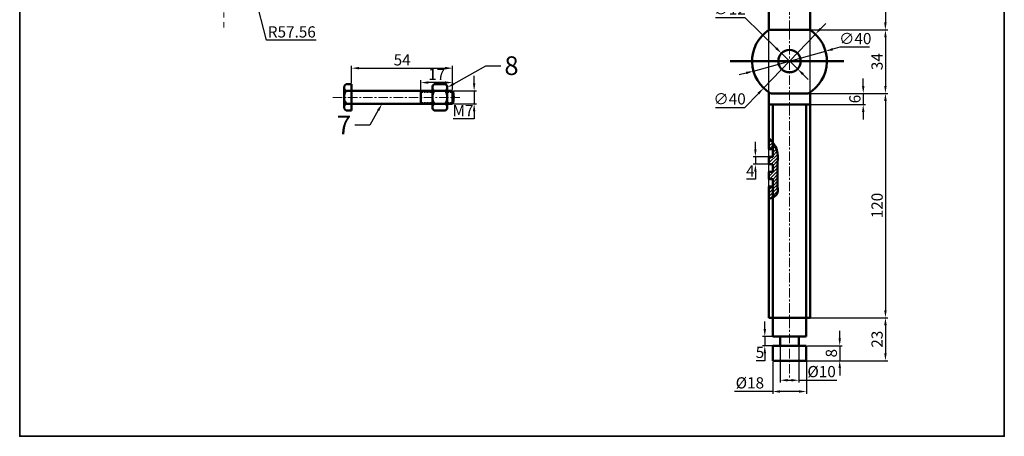
# Model space of a CAD drawing. Units: millimetres. Extents: x 44 to 571, y -292 to 291.
# Tile 1 of 4: x 44 to 571, y -292 to -69. Entities that reach past the tile are written whole.
import ezdxf
from ezdxf import colors
from ezdxf.entities.mleader import LeaderData, LeaderLine
from ezdxf.math import Vec2, Vec3

# ---------------------------------------------------------------- set-up
doc = ezdxf.new("R2010")
doc.units = ezdxf.units.MM
doc.header["$LTSCALE"] = 0.4
doc.linetypes.add('CENTER', pattern=[50.8, 31.75, -6.35, 6.35, -6.35])
doc.linetypes.add('HIDDEN', pattern=[9.525, 6.35, -3.175])
for name, color, linetype, lineweight in [('M-CNTR', 1, 'CENTER', 18), ('M-DIMS', 2, 'Continuous', 25), ('M-HATC', 8, 'Continuous', 18), ('M-HIDN', 3, 'HIDDEN', 25), ('M-OUTL', 7, 'Continuous', 50), ('M-TEXT', 3, 'Continuous', 25), ('M-TTLB', 7, 'Continuous', 35)]:
    doc.layers.add(name, color=color, linetype=linetype, lineweight=lineweight)
doc.styles.get("Standard").update_dxf_attribs({"font": 'arial.ttf'})
doc.dimstyles.new('ISO-25', dxfattribs={"dimtxt": 6, "dimasz": 4, "dimexe": 1.25, "dimexo": 0.625, "dimtad": 1, "dimtoh": 1, "dimdec": 0, "dimtxsty": 'Standard', "dimcen": 2.5, "dimadec": 0, "dimazin": 0, "dimtfac": 1, "dimtdec": 0, "dimtmove": 0, "dimatfit": 3, "dimfxl": 1, "dimarcsym": 0})

# ---------------------------------------------------------------- blocks, each defined once
blk = doc.blocks.new('*D53')
at = {"layer": 'Defpoints', "color": 0, "ltscale": 0.4, "transparency": 16777216}
for p in [(466.7, 205.39), (466.7, -74.61), (506.97, -74.61)]:
    blk.add_point(p, dxfattribs=at)
at = {"layer": 'M-DIMS', "color": 0, "lineweight": -2, "ltscale": 0.4, "transparency": 16777216}
for p, q in [((467.32, 205.39), (508.22, 205.39)), ((506.97, 201.39), (506.97, -70.61)), ((467.32, -74.61), (508.22, -74.61))]:
    blk.add_line(p, q, dxfattribs=at)
at = {"layer": 'M-DIMS', "color": 0, "ltscale": 0.4, "transparency": 16777216}
for points in [[(506.3, 201.39), (507.64, 201.39), (506.97, 205.39)], [(506.3, -70.61), (507.64, -70.61), (506.97, -74.61)]]:
    blk.add_solid(points, dxfattribs=at)
at = {"layer": 'M-DIMS', "color": 0, "ltscale": 0.4, "transparency": 16777216, "insert": (503.28, 65.39), "char_height": 6, "attachment_point": 5, "rotation": 90}
blk.add_mtext('280', dxfattribs=at)
blk = doc.blocks.new('*D54')
at = {"layer": 'Defpoints', "color": 0, "ltscale": 0.4, "transparency": 16777216}
for p in [(455.7, -74.61), (455.7, -108.61), (507, -108.61)]:
    blk.add_point(p, dxfattribs=at)
at = {"layer": 'M-DIMS', "color": 0, "lineweight": -2, "ltscale": 0.4, "transparency": 16777216}
for p, q in [((456.32, -74.61), (508.25, -74.61)), ((507, -78.61), (507, -104.61)), ((456.32, -108.61), (508.25, -108.61))]:
    blk.add_line(p, q, dxfattribs=at)
at = {"layer": 'M-DIMS', "color": 0, "ltscale": 0.4, "transparency": 16777216}
for points in [[(506.34, -78.61), (507.67, -78.61), (507, -74.61)], [(506.34, -104.61), (507.67, -104.61), (507, -108.61)]]:
    blk.add_solid(points, dxfattribs=at)
at = {"layer": 'M-DIMS', "color": 0, "ltscale": 0.4, "transparency": 16777216, "insert": (503.31, -91.61), "char_height": 6, "attachment_point": 5, "rotation": 90}
blk.add_mtext('34', dxfattribs=at)
blk = doc.blocks.new('*D55')
at = {"layer": 'Defpoints', "color": 0, "ltscale": 0.4, "transparency": 16777216}
for p in [(455.7, -108.61), (455.7, -114.61), (495.13, -114.61)]:
    blk.add_point(p, dxfattribs=at)
at = {"layer": 'M-DIMS', "color": 0, "lineweight": -2, "ltscale": 0.4, "transparency": 16777216}
for p, q in [((495.13, -104.61), (495.13, -100.61)), ((456.32, -108.61), (496.38, -108.61)), ((495.13, -108.61), (495.13, -114.61)), ((456.32, -114.61), (496.38, -114.61)), ((495.13, -118.61), (495.13, -122.61))]:
    blk.add_line(p, q, dxfattribs=at)
at = {"layer": 'M-DIMS', "color": 0, "ltscale": 0.4, "transparency": 16777216}
for points in [[(494.46, -104.61), (495.8, -104.61), (495.13, -108.61)], [(494.46, -118.61), (495.8, -118.61), (495.13, -114.61)]]:
    blk.add_solid(points, dxfattribs=at)
at = {"layer": 'M-DIMS', "color": 0, "ltscale": 0.4, "transparency": 16777216, "insert": (491.44, -111.61), "char_height": 6, "attachment_point": 5, "rotation": 90}
blk.add_mtext('6', dxfattribs=at)
blk = doc.blocks.new('*D56')
at = {"layer": 'Defpoints', "color": 0, "ltscale": 0.4, "transparency": 16777216}
for p in [(466.7, -108.61), (464.7, -228.61), (507, -228.61)]:
    blk.add_point(p, dxfattribs=at)
at = {"layer": 'M-DIMS', "color": 0, "lineweight": -2, "ltscale": 0.4, "transparency": 16777216}
for p, q in [((467.32, -108.61), (508.25, -108.61)), ((507, -112.61), (507, -224.61)), ((465.32, -228.61), (508.25, -228.61))]:
    blk.add_line(p, q, dxfattribs=at)
at = {"layer": 'M-DIMS', "color": 0, "ltscale": 0.4, "transparency": 16777216}
for points in [[(506.34, -112.61), (507.67, -112.61), (507, -108.61)], [(506.34, -224.61), (507.67, -224.61), (507, -228.61)]]:
    blk.add_solid(points, dxfattribs=at)
at = {"layer": 'M-DIMS', "color": 0, "ltscale": 0.4, "transparency": 16777216, "insert": (503.31, -168.61), "char_height": 6, "attachment_point": 5, "rotation": 90}
blk.add_mtext('120', dxfattribs=at)
blk = doc.blocks.new('*D57')
at = {"layer": 'Defpoints', "color": 0, "ltscale": 0.4, "transparency": 16777216}
for p in [(455.7, -228.61), (455.7, -251.61), (507, -251.61)]:
    blk.add_point(p, dxfattribs=at)
at = {"layer": 'M-DIMS', "color": 0, "lineweight": -2, "ltscale": 0.4, "transparency": 16777216}
for p, q in [((456.32, -228.61), (508.25, -228.61)), ((507, -232.61), (507, -247.61)), ((456.32, -251.61), (508.25, -251.61))]:
    blk.add_line(p, q, dxfattribs=at)
at = {"layer": 'M-DIMS', "color": 0, "ltscale": 0.4, "transparency": 16777216}
for points in [[(506.34, -232.61), (507.67, -232.61), (507, -228.61)], [(506.34, -247.61), (507.67, -247.61), (507, -251.61)]]:
    blk.add_solid(points, dxfattribs=at)
at = {"layer": 'M-DIMS', "color": 0, "ltscale": 0.4, "transparency": 16777216, "insert": (503.31, -240.11), "char_height": 6, "attachment_point": 5, "rotation": 90}
blk.add_mtext('23', dxfattribs=at)
blk = doc.blocks.new('*D58')
at = {"layer": 'Defpoints', "color": 0, "ltscale": 0.4, "transparency": 16777216}
for p in [(464.7, -243.61), (464.7, -251.61), (482.55, -251.61)]:
    blk.add_point(p, dxfattribs=at)
at = {"layer": 'M-DIMS', "color": 0, "lineweight": -2, "ltscale": 0.4, "transparency": 16777216}
for p, q in [((482.55, -239.61), (482.55, -235.61)), ((465.32, -243.61), (483.8, -243.61)), ((482.55, -243.61), (482.55, -251.61)), ((465.32, -251.61), (483.8, -251.61)), ((482.55, -255.61), (482.55, -259.61))]:
    blk.add_line(p, q, dxfattribs=at)
at = {"layer": 'M-DIMS', "color": 0, "ltscale": 0.4, "transparency": 16777216}
for points in [[(481.88, -239.61), (483.22, -239.61), (482.55, -243.61)], [(481.88, -255.61), (483.22, -255.61), (482.55, -251.61)]]:
    blk.add_solid(points, dxfattribs=at)
at = {"layer": 'M-DIMS', "color": 0, "ltscale": 0.4, "transparency": 16777216, "insert": (478.86, -247.61), "char_height": 6, "attachment_point": 5, "rotation": 90}
blk.add_mtext('8', dxfattribs=at)
blk = doc.blocks.new('*D59')
at = {"layer": 'Defpoints', "color": 0, "ltscale": 0.4, "transparency": 16777216}
for p in [(464.7, -238.61), (442.49, -243.61), (464.7, -243.61)]:
    blk.add_point(p, dxfattribs=at)
at = {"layer": 'M-DIMS', "color": 0, "lineweight": -2, "ltscale": 0.4, "transparency": 16777216}
for p, q in [((442.49, -234.61), (442.49, -230.61)), ((464.07, -238.61), (441.24, -238.61)), ((442.49, -238.61), (442.49, -243.61)), ((464.07, -243.61), (441.24, -243.61)), ((442.49, -251.61), (437.89, -251.61)), ((442.49, -247.61), (442.49, -251.61))]:
    blk.add_line(p, q, dxfattribs=at)
at = {"layer": 'M-DIMS', "color": 0, "ltscale": 0.4, "transparency": 16777216}
for points in [[(441.82, -234.61), (443.16, -234.61), (442.49, -238.61)], [(441.82, -247.61), (443.16, -247.61), (442.49, -243.61)]]:
    blk.add_solid(points, dxfattribs=at)
at = {"layer": 'M-DIMS', "color": 0, "ltscale": 0.4, "transparency": 16777216, "insert": (439.88, -247.94), "char_height": 6, "attachment_point": 5}
blk.add_mtext('5', dxfattribs=at)
blk = doc.blocks.new('*D60')
at = {"layer": 'Defpoints', "color": 0, "ltscale": 0.4, "transparency": 16777216}
for p in [(450.7, -243.61), (460.7, -243.61), (460.7, -262.09)]:
    blk.add_point(p, dxfattribs=at)
at = {"layer": 'M-DIMS', "color": 0, "lineweight": -2, "ltscale": 0.4, "transparency": 16777216}
for p, q in [((450.7, -244.24), (450.7, -263.34)), ((460.7, -244.24), (460.7, -263.34)), ((454.7, -262.09), (456.7, -262.09)), ((460.7, -262.09), (481.05, -262.09))]:
    blk.add_line(p, q, dxfattribs=at)
at = {"layer": 'M-DIMS', "color": 0, "ltscale": 0.4, "transparency": 16777216}
for points in [[(454.7, -261.42), (454.7, -262.75), (450.7, -262.09)], [(456.7, -261.42), (456.7, -262.75), (460.7, -262.09)]]:
    blk.add_solid(points, dxfattribs=at)
at = {"layer": 'M-DIMS', "color": 0, "ltscale": 0.4, "transparency": 16777216, "insert": (472.87, -258.23), "char_height": 6, "attachment_point": 5}
blk.add_mtext('%%C10', dxfattribs=at)
blk = doc.blocks.new('*D61')
at = {"layer": 'Defpoints', "color": 0, "ltscale": 0.4, "transparency": 16777216}
for p in [(446.7, -251.61), (464.7, -251.61), (464.7, -268.11)]:
    blk.add_point(p, dxfattribs=at)
at = {"layer": 'M-DIMS', "color": 0, "lineweight": -2, "ltscale": 0.4, "transparency": 16777216}
for p, q in [((446.7, -252.24), (446.7, -269.36)), ((464.7, -252.24), (464.7, -269.36)), ((446.7, -268.11), (426.31, -268.11)), ((460.7, -268.11), (450.7, -268.11))]:
    blk.add_line(p, q, dxfattribs=at)
at = {"layer": 'M-DIMS', "color": 0, "ltscale": 0.4, "transparency": 16777216}
for points in [[(450.7, -267.44), (450.7, -268.77), (446.7, -268.11)], [(460.7, -267.44), (460.7, -268.77), (464.7, -268.11)]]:
    blk.add_solid(points, dxfattribs=at)
at = {"layer": 'M-DIMS', "color": 0, "ltscale": 0.4, "transparency": 16777216, "insert": (434.5, -264.25), "char_height": 6, "attachment_point": 5}
blk.add_mtext('%%C18', dxfattribs=at)
blk = doc.blocks.new('*D62')
at = {"layer": 'Defpoints', "color": 0, "ltscale": 0.4, "transparency": 16777216}
for p in [(474.98, -86.01), (436.41, -96.62)]:
    blk.add_point(p, dxfattribs=at)
at = {"layer": 'M-DIMS', "color": 0, "lineweight": -2, "ltscale": 0.4, "transparency": 16777216}
for p, q in [((482.69, -83.89), (478.84, -84.95)), ((498.42, -83.89), (482.69, -83.89)), ((436.41, -96.62), (474.98, -86.01)), ((432.55, -97.68), (428.7, -98.74))]:
    blk.add_line(p, q, dxfattribs=at)
at = {"layer": 'M-DIMS', "color": 0, "ltscale": 0.4, "transparency": 16777216}
for points in [[(478.66, -84.31), (479.01, -85.6), (474.98, -86.01)], [(432.38, -97.03), (432.73, -98.32), (436.41, -96.62)]]:
    blk.add_solid(points, dxfattribs=at)
at = {"layer": 'M-DIMS', "color": 0, "ltscale": 0.4, "transparency": 16777216, "insert": (490.87, -80.04), "char_height": 6, "attachment_point": 5}
blk.add_mtext('∅40', dxfattribs=at)
blk = doc.blocks.new('*D63')
at = {"layer": 'Defpoints', "color": 0, "ltscale": 0.4, "transparency": 16777216}
for p in [(451.4, -87.13), (460, -95.5)]:
    blk.add_point(p, dxfattribs=at)
at = {"layer": 'M-DIMS', "color": 0, "lineweight": -2, "ltscale": 0.4, "transparency": 16777216}
for p, q in [((416.09, -68.05), (431.77, -68.05)), ((431.77, -68.05), (448.53, -84.34)), ((460, -95.5), (451.4, -87.13)), ((462.86, -98.29), (465.73, -101.08))]:
    blk.add_line(p, q, dxfattribs=at)
at = {"layer": 'M-DIMS', "color": 0, "ltscale": 0.4, "transparency": 16777216}
for points in [[(448.99, -83.86), (448.06, -84.82), (451.4, -87.13)], [(463.33, -97.81), (462.4, -98.76), (460, -95.5)]]:
    blk.add_solid(points, dxfattribs=at)
at = {"layer": 'M-DIMS', "color": 0, "ltscale": 0.4, "transparency": 16777216, "insert": (423.62, -64.19), "char_height": 6, "attachment_point": 5}
blk.add_mtext('∅12', dxfattribs=at)
blk = doc.blocks.new('*D64')
at = {"layer": 'Defpoints', "color": 0, "ltscale": 0.4, "transparency": 16777216}
for p in [(437.46, -146.49), (444.7, -142.49), (444.7, -146.49)]:
    blk.add_point(p, dxfattribs=at)
at = {"layer": 'M-DIMS', "color": 0, "lineweight": -2, "ltscale": 0.4, "transparency": 16777216}
for p, q in [((437.46, -138.49), (437.46, -134.49)), ((444.07, -142.49), (436.21, -142.49)), ((444.07, -146.49), (436.21, -146.49)), ((437.46, -142.49), (437.46, -146.49)), ((437.46, -150.49), (437.46, -154.49)), ((437.46, -154.49), (432.68, -154.49))]:
    blk.add_line(p, q, dxfattribs=at)
at = {"layer": 'M-DIMS', "color": 0, "ltscale": 0.4, "transparency": 16777216}
for points in [[(436.79, -138.49), (438.12, -138.49), (437.46, -142.49)], [(436.79, -150.49), (438.12, -150.49), (437.46, -146.49)]]:
    blk.add_solid(points, dxfattribs=at)
at = {"layer": 'M-DIMS', "color": 0, "ltscale": 0.4, "transparency": 16777216, "insert": (434.76, -150.87), "char_height": 6, "attachment_point": 5}
blk.add_mtext('4', dxfattribs=at)
blk = doc.blocks.new('*D71')
at = {"layer": 'Defpoints', "color": 0, "ltscale": 0.4, "transparency": 16777216}
for p in [(275.56, -95.1), (221.56, -103.69), (275.56, -107.19)]:
    blk.add_point(p, dxfattribs=at)
at = {"layer": 'M-DIMS', "color": 0, "lineweight": -2, "ltscale": 0.4, "transparency": 16777216}
for p, q in [((221.56, -103.06), (221.56, -93.85)), ((275.56, -106.56), (275.56, -93.85)), ((225.56, -95.1), (271.56, -95.1))]:
    blk.add_line(p, q, dxfattribs=at)
at = {"layer": 'M-DIMS', "color": 0, "ltscale": 0.4, "transparency": 16777216}
for points in [[(225.56, -94.44), (225.56, -95.77), (221.56, -95.1)], [(271.56, -94.44), (271.56, -95.77), (275.56, -95.1)]]:
    blk.add_solid(points, dxfattribs=at)
at = {"layer": 'M-DIMS', "color": 0, "ltscale": 0.4, "transparency": 16777216, "insert": (248.56, -91.43), "char_height": 6, "attachment_point": 5}
blk.add_mtext('54', dxfattribs=at)
blk = doc.blocks.new('*D72')
at = {"layer": 'Defpoints', "color": 0, "ltscale": 0.4, "transparency": 16777216}
for p in [(258.56, -102.8), (258.56, -107.19), (275.56, -107.19)]:
    blk.add_point(p, dxfattribs=at)
at = {"layer": 'M-DIMS', "color": 0, "lineweight": -2, "ltscale": 0.4, "transparency": 16777216}
for p, q in [((258.56, -106.56), (258.56, -101.55)), ((271.56, -102.8), (262.56, -102.8)), ((275.56, -106.56), (275.56, -101.55))]:
    blk.add_line(p, q, dxfattribs=at)
at = {"layer": 'M-DIMS', "color": 0, "ltscale": 0.4, "transparency": 16777216}
for points in [[(262.56, -102.14), (262.56, -103.47), (258.56, -102.8)], [(271.56, -102.14), (271.56, -103.47), (275.56, -102.8)]]:
    blk.add_solid(points, dxfattribs=at)
at = {"layer": 'M-DIMS', "color": 0, "ltscale": 0.4, "transparency": 16777216, "insert": (267.06, -99.16), "char_height": 6, "attachment_point": 5}
blk.add_mtext('17', dxfattribs=at)
blk = doc.blocks.new('*D73')
at = {"layer": 'Defpoints', "color": 0, "ltscale": 0.4, "transparency": 16777216}
for p in [(275.56, -107.19), (275.56, -114.19), (287.06, -114.19)]:
    blk.add_point(p, dxfattribs=at)
at = {"layer": 'M-DIMS', "color": 0, "lineweight": -2, "ltscale": 0.4, "transparency": 16777216}
for p, q in [((287.06, -103.19), (287.06, -99.19)), ((276.18, -107.19), (288.31, -107.19)), ((287.06, -107.19), (287.06, -114.19)), ((276.18, -114.19), (288.31, -114.19)), ((287.06, -118.19), (287.06, -122.19)), ((287.06, -122.19), (275.8, -122.19))]:
    blk.add_line(p, q, dxfattribs=at)
at = {"layer": 'M-DIMS', "color": 0, "ltscale": 0.4, "transparency": 16777216}
for points in [[(286.4, -103.19), (287.73, -103.19), (287.06, -107.19)], [(286.4, -118.19), (287.73, -118.19), (287.06, -114.19)]]:
    blk.add_solid(points, dxfattribs=at)
at = {"layer": 'M-DIMS', "color": 0, "ltscale": 0.4, "transparency": 16777216, "insert": (281.12, -118.56), "char_height": 6, "attachment_point": 5}
blk.add_mtext('M7', dxfattribs=at)
blk = doc.blocks.new('*D77')
at = {"layer": 'Defpoints', "color": 0, "ltscale": 0.4, "transparency": 16777216}
for p in [(466.7, 250.52), (444.7, -228.61), (466.7, -228.61)]:
    blk.add_point(p, dxfattribs=at)
at = {"layer": 'M-DIMS', "color": 0, "lineweight": -2, "ltscale": 0.4, "transparency": 16777216}
for p, q in [((444.7, -227.99), (444.7, 251.77)), ((448.7, 250.52), (462.7, 250.52)), ((466.7, -227.99), (466.7, 251.77))]:
    blk.add_line(p, q, dxfattribs=at)
at = {"layer": 'M-DIMS', "color": 0, "ltscale": 0.4, "transparency": 16777216}
for points in [[(448.7, 251.19), (448.7, 249.85), (444.7, 250.52)], [(462.7, 251.19), (462.7, 249.85), (466.7, 250.52)]]:
    blk.add_solid(points, dxfattribs=at)
at = {"layer": 'M-DIMS', "color": 0, "ltscale": 0.4, "transparency": 16777216, "insert": (455.7, 254.16), "char_height": 6, "attachment_point": 5}
blk.add_mtext('22', dxfattribs=at)
blk = doc.blocks.new('*D81')
at = {"layer": 'Defpoints', "color": 0, "ltscale": 0.4, "transparency": 16777216}
for p in [(153.17, 9.08), (167.4, -46.7)]:
    blk.add_point(p, dxfattribs=at)
at = {"layer": 'M-DIMS', "color": 0, "lineweight": -2, "ltscale": 0.4, "transparency": 16777216}
for p, q in [((153.17, 9.08), (167.4, -46.7)), ((175.94, -80.16), (168.39, -50.57)), ((202.55, -80.16), (175.94, -80.16))]:
    blk.add_line(p, q, dxfattribs=at)
at = {"layer": 'M-DIMS', "color": 0, "ltscale": 0.4, "transparency": 16777216}
blk.add_solid([(169.03, -50.41), (167.74, -50.74), (167.4, -46.7)], dxfattribs=at)
at = {"layer": 'M-DIMS', "color": 0, "ltscale": 0.4, "transparency": 16777216, "insert": (189.55, -76.47), "char_height": 6, "attachment_point": 5}
blk.add_mtext('R57.56', dxfattribs=at)
blk = doc.blocks.new('*D85')
at = {"layer": 'Defpoints', "color": 0, "ltscale": 0.4, "transparency": 16777216}
for p in [(469.55, -76.89), (441.85, -105.74)]:
    blk.add_point(p, dxfattribs=at)
at = {"layer": 'M-DIMS', "color": 0, "lineweight": -2, "ltscale": 0.4, "transparency": 16777216}
for p, q in [((472.32, -74), (475.09, -71.12)), ((469.55, -76.89), (441.85, -105.74)), ((431.83, -116.18), (439.08, -108.63)), ((416.1, -116.18), (431.83, -116.18))]:
    blk.add_line(p, q, dxfattribs=at)
at = {"layer": 'M-DIMS', "color": 0, "ltscale": 0.4, "transparency": 16777216}
for points in [[(471.84, -73.54), (472.8, -74.46), (469.55, -76.89)], [(438.6, -108.17), (439.56, -109.09), (441.85, -105.74)]]:
    blk.add_solid(points, dxfattribs=at)
at = {"layer": 'M-DIMS', "color": 0, "ltscale": 0.4, "transparency": 16777216, "insert": (423.66, -112.32), "char_height": 6, "attachment_point": 5}
blk.add_mtext('∅40', dxfattribs=at)

msp = doc.modelspace()

# ---------------------------------------------------------------- hatches: boundary and pattern name
at = {"layer": 'M-HATC', "ltscale": 0.4}
h = msp.add_hatch(dxfattribs=at)
h.set_pattern_fill('ANSI31', color=256, scale=0.4)
h.set_pattern_definition([(45, (-76.2027, 76.8526), (-0.8980256, 0.8980256), [])])
edge = h.paths.add_edge_path()
edge.add_spline(control_points=[(449.311, -146.8439), (449.3105, -146.3114), (449.3256, -144.8584), (449.4232, -143.3994), (449.4254, -142.4776)], knot_values=[11.32328929, 11.32328929, 11.32328929, 11.32328929, 12.92212287, 15.6865182, 15.6865182, 15.6865182, 15.6865182], degree=3, periodic=0)
edge.add_spline(control_points=[(449.4254, -142.4776), (449.4263, -142.1195), (449.4182, -141.7617), (449.3957, -141.4046)], knot_values=[10.24928519, 10.24928519, 10.24928519, 10.24928519, 11.32328929, 11.32328929, 11.32328929, 11.32328929], degree=3, periodic=0)
edge.add_spline(control_points=[(449.3957, -141.4046), (449.3811, -141.1744), (449.3497, -140.8226), (449.3009, -140.4716), (449.2819, -140.3501)], knot_values=[9.18976333, 9.18976333, 9.18976333, 9.18976333, 9.88210686, 10.24928519, 10.24928519, 10.24928519, 10.24928519], degree=3, periodic=0)
edge.add_spline(control_points=[(449.2819, -140.3501), (449.2387, -140.0745), (449.1849, -139.7999), (449.1206, -139.5275)], knot_values=[8.35630379, 8.35630379, 8.35630379, 8.35630379, 9.18976333, 9.18976333, 9.18976333, 9.18976333], degree=3, periodic=0)
edge.add_spline(control_points=[(449.1206, -139.5275), (449.0768, -139.3419), (449.0282, -139.1572), (448.9747, -138.9741)], knot_values=[7.78801385, 7.78801385, 7.78801385, 7.78801385, 8.35630379, 8.35630379, 8.35630379, 8.35630379], degree=3, periodic=0)
edge.add_spline(control_points=[(448.9747, -138.9741), (448.883, -138.6597), (448.7773, -138.3495), (448.6579, -138.0456)], knot_values=[6.8125257, 6.8125257, 6.8125257, 6.8125257, 7.78801385, 7.78801385, 7.78801385, 7.78801385], degree=3, periodic=0)
edge.add_spline(control_points=[(448.6579, -138.0456), (448.5803, -137.8482), (448.497, -137.6534), (448.408, -137.4618)], knot_values=[6.17878041, 6.17878041, 6.17878041, 6.17878041, 6.8125257, 6.8125257, 6.8125257, 6.8125257], degree=3, periodic=0)
edge.add_spline(control_points=[(448.408, -137.4618), (448.3704, -137.3808), (448.2904, -137.2143), (448.2062, -137.0504), (448.1616, -136.9663)], knot_values=[5.62420852, 5.62420852, 5.62420852, 5.62420852, 5.89215571, 6.17878041, 6.17878041, 6.17878041, 6.17878041], degree=3, periodic=0)
edge.add_spline(control_points=[(448.1616, -136.9663), (448.0006, -136.6632), (447.8255, -136.3686), (447.6388, -136.0811)], knot_values=[4.59032808, 4.59032808, 4.59032808, 4.59032808, 5.62420852, 5.62420852, 5.62420852, 5.62420852], degree=3, periodic=0)
edge.add_spline(control_points=[(447.6388, -136.0811), (447.4828, -135.8408), (447.3187, -135.6054), (447.148, -135.374)], knot_values=[3.7261445, 3.7261445, 3.7261445, 3.7261445, 4.59032808, 4.59032808, 4.59032808, 4.59032808], degree=3, periodic=0)
edge.add_spline(control_points=[(447.148, -135.374), (447.0019, -135.176), (446.8511, -134.9809), (446.6963, -134.7881)], knot_values=[2.98657145, 2.98657145, 2.98657145, 2.98657145, 3.7261445, 3.7261445, 3.7261445, 3.7261445], degree=3, periodic=0)
edge.add_line((446.6963, -134.7881), (446.6963, -142.4919))
edge.add_line((446.6963, -142.4919), (444.6963, -142.4919))
edge.add_line((444.6963, -142.4919), (444.6963, -146.4919))
edge.add_line((444.6963, -146.4919), (446.6963, -146.4919))
edge.add_line((446.6963, -146.4919), (446.6963, -150.4919))
edge.add_line((446.6963, -150.4919), (444.6963, -150.4919))
edge.add_line((444.6963, -150.4919), (444.6963, -154.4919))
edge.add_line((444.6963, -154.4919), (446.6963, -154.4919))
edge.add_line((446.6963, -154.4919), (446.6963, -164.2354))
edge.add_spline(control_points=[(446.6963, -164.2354), (446.7656, -164.2027), (446.8343, -164.1696), (446.9021, -164.1361)], knot_values=[34.24926087, 34.24926087, 34.24926087, 34.24926087, 34.45620414, 34.45620414, 34.45620414, 34.45620414], degree=3, periodic=0)
edge.add_spline(control_points=[(446.9021, -164.1361), (447.1117, -164.0326), (447.314, -163.9253), (447.5067, -163.813)], knot_values=[33.60988749, 33.60988749, 33.60988749, 33.60988749, 34.24926087, 34.24926087, 34.24926087, 34.24926087], degree=3, periodic=0)
edge.add_spline(control_points=[(447.5067, -163.813), (447.7529, -163.6694), (447.9835, -163.5177), (448.1937, -163.3553)], knot_values=[32.79282131, 32.79282131, 32.79282131, 32.79282131, 33.60988749, 33.60988749, 33.60988749, 33.60988749], degree=3, periodic=0)
edge.add_spline(control_points=[(448.1937, -163.3553), (448.2605, -163.3037), (448.3252, -163.2511), (448.3876, -163.1973)], knot_values=[32.53342587, 32.53342587, 32.53342587, 32.53342587, 32.79282131, 32.79282131, 32.79282131, 32.79282131], degree=3, periodic=0)
edge.add_spline(control_points=[(448.3876, -163.1973), (448.4564, -163.1381), (448.5224, -163.0776), (448.5856, -163.0155)], knot_values=[32.24811052, 32.24811052, 32.24811052, 32.24811052, 32.53342587, 32.53342587, 32.53342587, 32.53342587], degree=3, periodic=0)
edge.add_spline(control_points=[(448.5856, -163.0155), (448.6429, -162.9593), (448.6979, -162.9018), (448.7503, -162.8431)], knot_values=[31.98952685, 31.98952685, 31.98952685, 31.98952685, 32.24811052, 32.24811052, 32.24811052, 32.24811052], degree=3, periodic=0)
edge.add_spline(control_points=[(448.7503, -162.8431), (448.8083, -162.778), (448.8632, -162.7114), (448.9149, -162.643)], knot_values=[31.70339974, 31.70339974, 31.70339974, 31.70339974, 31.98952685, 31.98952685, 31.98952685, 31.98952685], degree=3, periodic=0)
edge.add_spline(control_points=[(448.9149, -162.643), (448.9615, -162.5814), (449.0055, -162.5184), (449.0466, -162.4539)], knot_values=[31.44544701, 31.44544701, 31.44544701, 31.44544701, 31.70339974, 31.70339974, 31.70339974, 31.70339974], degree=3, periodic=0)
edge.add_spline(control_points=[(449.0466, -162.4539), (449.0819, -162.3986), (449.1152, -162.3422), (449.1463, -162.2846)], knot_values=[31.22405118, 31.22405118, 31.22405118, 31.22405118, 31.44544701, 31.44544701, 31.44544701, 31.44544701], degree=3, periodic=0)
edge.add_spline(control_points=[(449.1463, -162.2846), (449.1817, -162.219), (449.2144, -162.1519), (449.2441, -162.0833)], knot_values=[30.97154718, 30.97154718, 30.97154718, 30.97154718, 31.22405118, 31.22405118, 31.22405118, 31.22405118], degree=3, periodic=0)
edge.add_spline(control_points=[(449.2441, -162.0833), (449.2607, -162.0449), (449.2764, -162.006), (449.2912, -161.9667)], knot_values=[30.83030721, 30.83030721, 30.83030721, 30.83030721, 30.97154718, 30.97154718, 30.97154718, 30.97154718], degree=3, periodic=0)
edge.add_spline(control_points=[(449.2912, -161.9667), (449.306, -161.9272), (449.3263, -161.8685), (449.3445, -161.8086), (449.3502, -161.7893)], knot_values=[30.62215627, 30.62215627, 30.62215627, 30.62215627, 30.76364572, 30.83030721, 30.83030721, 30.83030721, 30.83030721], degree=3, periodic=0)
edge.add_spline(control_points=[(449.3502, -161.7893), (449.3725, -161.7129), (449.3915, -161.6348), (449.4076, -161.5551)], knot_values=[30.35787543, 30.35787543, 30.35787543, 30.35787543, 30.62215627, 30.62215627, 30.62215627, 30.62215627], degree=3, periodic=0)
edge.add_spline(control_points=[(449.4076, -161.5551), (449.4241, -161.4728), (449.4375, -161.3889), (449.4482, -161.3036)], knot_values=[30.08521848, 30.08521848, 30.08521848, 30.08521848, 30.35787543, 30.35787543, 30.35787543, 30.35787543], degree=3, periodic=0)
edge.add_spline(control_points=[(449.4482, -161.3036), (449.4638, -161.1785), (449.4734, -161.0503), (449.4783, -160.9196)], knot_values=[29.68546604, 29.68546604, 29.68546604, 29.68546604, 30.08521848, 30.08521848, 30.08521848, 30.08521848], degree=3, periodic=0)
edge.add_spline(control_points=[(449.4783, -160.9196), (449.4854, -160.7292), (449.4823, -160.5335), (449.4729, -160.3344)], knot_values=[29.10320055, 29.10320055, 29.10320055, 29.10320055, 29.68546604, 29.68546604, 29.68546604, 29.68546604], degree=3, periodic=0)
edge.add_spline(control_points=[(449.4729, -160.3344), (449.4624, -160.1131), (449.444, -159.8876), (449.4227, -159.6606)], knot_values=[28.45564578, 28.45564578, 28.45564578, 28.45564578, 29.10320055, 29.10320055, 29.10320055, 29.10320055], degree=3, periodic=0)
edge.add_spline(control_points=[(449.4227, -159.6606), (449.3937, -159.3513), (449.1492, -157.1274), (449.3114, -154.7841), (449.3462, -152.6616), (449.3495, -152.3282)], knot_values=[21.16302827, 21.16302827, 21.16302827, 21.16302827, 22.0455532, 27.45206686, 28.45564578, 28.45564578, 28.45564578, 28.45564578], degree=3, periodic=0)
edge.add_spline(control_points=[(449.3495, -152.3282), (449.3545, -151.8289), (449.3548, -151.3272), (449.3521, -150.8246)], knot_values=[19.66000263, 19.66000263, 19.66000263, 19.66000263, 21.16302827, 21.16302827, 21.16302827, 21.16302827], degree=3, periodic=0)
edge.add_spline(control_points=[(449.3521, -150.8246), (449.3489, -150.2049), (449.3325, -148.8736), (449.3116, -147.5499), (449.311, -146.8439)], knot_values=[15.6865182, 15.6865182, 15.6865182, 15.6865182, 17.54010114, 19.66000263, 19.66000263, 19.66000263, 19.66000263], degree=3, periodic=0)
edge = h.paths.add_edge_path()
edge.add_spline(control_points=[(446.6963, -134.7881), (446.0715, -134.0097), (445.3839, -133.2694), (444.6963, -132.5292)], knot_values=[0, 0, 0, 0, 2.98657145, 2.98657145, 2.98657145, 2.98657145], degree=3, periodic=0)
edge.add_line((444.6963, -132.5292), (444.6963, -138.4919))
edge.add_line((444.6963, -138.4919), (446.6963, -138.4919))
edge.add_line((446.6963, -138.4919), (446.6963, -134.7881))
edge = h.paths.add_edge_path()
edge.add_line((446.6963, -158.4919), (444.6963, -158.4919))
edge.add_line((444.6963, -158.4919), (444.6963, -165.0665))
edge.add_spline(control_points=[(444.6963, -165.0665), (445.0158, -164.9421), (445.3353, -164.8176), (445.649, -164.6902)], knot_values=[35.45876189, 35.45876189, 35.45876189, 35.45876189, 36.33344142, 36.33344142, 36.33344142, 36.33344142], degree=3, periodic=0)
edge.add_spline(control_points=[(445.649, -164.6902), (445.726, -164.6589), (445.8027, -164.6274), (445.8789, -164.5957)], knot_values=[35.24401985, 35.24401985, 35.24401985, 35.24401985, 35.45876189, 35.45876189, 35.45876189, 35.45876189], degree=3, periodic=0)
edge.add_spline(control_points=[(445.8789, -164.5957), (445.9597, -164.5621), (446.0401, -164.5282), (446.1198, -164.4941)], knot_values=[35.0163632, 35.0163632, 35.0163632, 35.0163632, 35.24401985, 35.24401985, 35.24401985, 35.24401985], degree=3, periodic=0)
edge.add_spline(control_points=[(446.1198, -164.4941), (446.3161, -164.41), (446.5087, -164.324), (446.6963, -164.2354)], knot_values=[34.45620383, 34.45620383, 34.45620383, 34.45620383, 35.0163632, 35.0163632, 35.0163632, 35.0163632], degree=3, periodic=0)
edge.add_line((446.6963, -164.2354), (446.6963, -158.4919))

# ---------------------------------------------------------------- linework, layer by layer
at = {"layer": 'M-CNTR', "ltscale": 0.4}
for p, q in [((455.6963, -74.6115), (455.6963, 225.3706)), ((455.6963, -74.6115), (455.6963, -260.9021)), ((211.4444, -110.7266), (279.4867, -110.7266))]:
    msp.add_line(p, q, dxfattribs=at)
at = {"layer": 'M-CNTR'}
msp.add_line((153.1682, 153.0761), (153.1682, -73.3053), dxfattribs=at)
at = {"layer": 'M-HIDN', "ltscale": 0.4}
for p, q in [((258.556, -107.9362), (264.7047, -107.9362)), ((272.7047, -107.9362), (275.556, -107.9362)), ((258.556, -113.4362), (264.7047, -113.4362)), ((272.7047, -113.4362), (275.556, -113.4362))]:
    msp.add_line(p, q, dxfattribs=at)
at = {"layer": 'M-OUTL', "ltscale": 0.4}
for p, q in [((444.6963, -74.6115), (444.6963, 51.668)), ((466.6963, 51.668), (466.6963, -74.6115)), ((444.6963, -74.6115), (466.6963, -74.6115)), ((444.6963, -74.6115), (466.6963, -74.6115)), ((484.7556, -91.3148), (423.9803, -91.3148)), ((218.556, -103.6862), (221.556, -103.6862)), ((221.556, -103.6862), (221.556, -117.6862)), ((265.7047, -103.6862), (271.7047, -103.6862)), ((217.556, -116.0349), (217.556, -105.4183)), ((221.556, -107.1862), (218.556, -107.1862)), ((221.556, -107.1862), (275.556, -107.1862)), ((258.556, -107.1862), (258.556, -114.1862)), ((264.7047, -116.0349), (264.7047, -105.4183)), ((271.7047, -107.1862), (265.7047, -107.1862)), ((272.7047, -105.4183), (272.7047, -116.0349)), ((272.7047, -116.0349), (272.7047, -105.4183)), ((275.556, -107.1862), (275.556, -114.1862)), ((444.6963, -138.4919), (444.6963, -108.0181)), ((445.6552, -108.6115), (465.7374, -108.6115)), ((466.6963, -228.6115), (466.6963, -108.0181)), ((221.556, -114.1862), (218.556, -114.1862)), ((275.556, -114.1862), (221.556, -114.1862)), ((271.7047, -114.1862), (265.7047, -114.1862)), ((444.6963, -114.6115), (466.6963, -114.6115)), ((446.6963, -142.4919), (446.6963, -114.6115)), ((464.6963, -238.6115), (464.6963, -114.6115)), ((221.556, -117.6862), (218.556, -117.6862)), ((271.7047, -117.6862), (265.7047, -117.6862)), ((444.6963, -138.4919), (446.6963, -138.4919)), ((444.6963, -142.4919), (446.6963, -142.4919)), ((444.6963, -146.4919), (444.6963, -142.4919)), ((446.6963, -146.4919), (444.6963, -146.4919)), ((446.6963, -150.4919), (446.6963, -146.4919)), ((444.6963, -150.4919), (446.6963, -150.4919)), ((444.6963, -154.4919), (444.6963, -150.4919)), ((446.6963, -154.4919), (444.6963, -154.4919)), ((446.6963, -228.6115), (446.6963, -154.4919)), ((444.6963, -228.6115), (444.6963, -158.4919)), ((444.6963, -158.4919), (446.6963, -158.4919)), ((444.6963, -228.6115), (466.6963, -228.6115)), ((446.6963, -228.6115), (446.6963, -238.6115)), ((464.6963, -228.6115), (464.6963, -238.6115)), ((464.6963, -238.6115), (446.6963, -238.6115)), ((450.6963, -238.6115), (450.6963, -243.6115)), ((460.6963, -243.6115), (460.6963, -238.6115)), ((464.6963, -243.6115), (446.6963, -243.6115)), ((446.6963, -243.6115), (446.6963, -251.6115)), ((464.6963, -251.6115), (464.6963, -243.6115)), ((446.6963, -251.6115), (464.6963, -251.6115))]:
    msp.add_line(p, q, dxfattribs=at)
msp.add_circle((455.6963, -91.3148), 6, dxfattribs=at)
for centre, radius, start, end in [((455.6963, -91.3148), 20, 123.367013, 239.863909), ((455.6963, -91.3148), 20, 300.136091, 56.632987), ((219.5871, -105.4362), 2.0312, 120.506323, 239.493677), ((266.7358, -105.4362), 2.0312, 120.506323, 239.493677), ((270.6737, -105.4362), 2.0312, 300.506323, 59.493677), ((224.181, -110.6862), 6.625, 148.109208, 211.890792), ((271.3297, -110.6862), 6.625, 148.109208, 211.890792), ((266.0797, -110.6862), 6.625, 328.109208, 31.890792), ((265.0729, -110.6862), 11.052, 341.537425, 18.462575), ((219.5824, -115.9362), 2.0288, 120.391765, 239.608235), ((266.7311, -115.9362), 2.0288, 120.391765, 239.608235), ((270.6784, -115.9362), 2.0288, 300.391765, 59.608235)]:
    msp.add_arc(centre, radius, start, end, dxfattribs=at)
msp.add_open_spline([(444.6963, -132.5292), (446.0572, -133.9942), (448.2575, -136.363), (449.6252, -140.9961), (449.2681, -144.9802), (449.3403, -149.1709), (449.3861, -153.7055), (449.0995, -157.845), (449.9577, -163.017), (446.758, -164.2634), (444.6963, -165.0665)], degree=3, knots=[0, 0, 0, 0, 5.91083322, 9.55694166, 14.08768462, 17.80641968, 22.1666072, 27.57312085, 30.68881776, 36.33344142, 36.33344142, 36.33344142, 36.33344142], dxfattribs=at)
at = {"layer": 'M-TTLB', "ltscale": 0.4}
msp.add_lwpolyline([(44.037, 291.1069), (570.566, 291.1069), (570.566, -292.0762), (44.037, -292.0762)], close=True, dxfattribs=at)

# ---------------------------------------------------------------- dimensions: what is measured, and where the dimension line sits
at = {"layer": 'M-DIMS', "ltscale": 0.4}
for base, p1, p2, override, picture, middle in [((466.6963, 250.5206), (444.6963, -228.6115), (466.6963, -228.6115), {"dimdec": 0, "dimlfac": 1, "dimrnd": 0, "dimzin": 0, "dimdsep": 46, "dimlunit": 2}, '*D77', (455.6963, 254.1579)), ((275.556, -95.1046), (221.556, -103.6862), (275.556, -107.1862), {"dimclrd": 0, "dimclre": 0, "dimclrt": 0}, '*D71', (248.556, -91.4285)), ((258.556, -102.8017), (275.556, -107.1862), (258.556, -107.1862), {"dimclrd": 0, "dimclre": 0, "dimclrt": 0}, '*D72', (267.056, -99.1645))]:
    dim = msp.add_linear_dim(base=base, p1=p1, p2=p2, dimstyle='ISO-25', override=override, dxfattribs=at)
    dim.commit()
    dim.dimension.update_dxf_attribs({"geometry": picture, "text_midpoint": middle})
for base, p1, p2, picture, middle in [((506.9684, -74.6115), (466.6963, 205.3885), (466.6963, -74.6115), '*D53', (503.2799, 65.3885)), ((507.0021, -108.6115), (455.6963, -74.6115), (455.6963, -108.6115), '*D54', (503.3117, -91.6115)), ((507.0021, -228.6115), (466.6963, -108.6115), (464.6963, -228.6115), '*D56', (503.3137, -168.6115)), ((437.4583, -146.4919), (444.6963, -142.4919), (444.6963, -146.4919), '*D64', (434.7583, -150.8669)), ((442.4902, -243.6115), (464.6963, -238.6115), (464.6963, -243.6115), '*D59', (439.8761, -247.9354)), ((507.0021, -251.6115), (455.6963, -228.6115), (455.6963, -251.6115), '*D57', (503.3117, -240.1115)), ((482.5511, -251.6115), (464.6963, -243.6115), (464.6963, -251.6115), '*D58', (478.8627, -247.6115))]:
    dim = msp.add_linear_dim(base=base, p1=p1, p2=p2, angle=90, dimstyle='ISO-25', override={"dimclrd": 0, "dimclre": 0, "dimclrt": 0}, dxfattribs=at)
    dim.commit()
    dim.dimension.update_dxf_attribs({"geometry": picture, "text_midpoint": middle})
dim = msp.add_radius_dim(center=(153.1682, 9.0761), mpoint=(167.398, -46.6959), dimstyle='ISO-25', override={"dimdec": 2, "dimlfac": 1, "dimrnd": 0, "dimzin": 0, "dimdsep": 46, "dimlunit": 2}, dxfattribs=at)
dim.commit()
dim.dimension.update_dxf_attribs({"geometry": '*D81', "text_midpoint": (189.5533, -80.1591), "dimtype": 164})
for p1, p2, override, picture, middle in [((459.9974, -95.4982), (451.3952, -87.1315), {"dimclrd": 0, "dimclre": 0, "dimclrt": 0}, '*D63', (423.6163, -68.0455)), ((469.5462, -76.8864), (441.8464, -105.7433), {"dimdec": 0, "dimlfac": 1, "dimrnd": 0, "dimzin": 0, "dimdsep": 46, "dimlunit": 2}, '*D85', (423.6551, -116.1768))]:
    dim = msp.add_diameter_dim_2p(p1=p1, p2=p2, dimstyle='ISO-25', override=override, dxfattribs=at)
    dim.commit()
    dim.dimension.update_dxf_attribs({"geometry": picture, "text_midpoint": middle, "dimtype": 163})
dim = msp.add_diameter_dim_2p(p1=(436.4117, -96.6162), p2=(474.9809, -86.0135), dimstyle='ISO-25', override={"dimclrd": 0, "dimclre": 0, "dimclrt": 0}, dxfattribs=at)
dim.commit()
dim.dimension.update_dxf_attribs({"geometry": '*D62', "text_midpoint": (490.8709, -80.0367)})
dim = msp.add_linear_dim(base=(287.0634, -114.1862), p1=(275.556, -107.1862), p2=(275.556, -114.1862), angle=90, text='M<>', dimstyle='ISO-25', override={"dimclrd": 0, "dimclre": 0, "dimclrt": 0}, dxfattribs=at)
dim.commit()
dim.dimension.update_dxf_attribs({"geometry": '*D73', "text_midpoint": (281.1178, -118.5612)})
dim = msp.add_linear_dim(base=(495.129, -114.6115), p1=(455.6963, -108.6115), p2=(455.6963, -114.6115), angle=90, dimstyle='ISO-25', override={"dimclrd": 0, "dimclre": 0, "dimclrt": 0}, dxfattribs=at)
dim.commit()
dim.dimension.update_dxf_attribs({"geometry": '*D55', "text_midpoint": (495.129, -111.6115), "dimtype": 160})
dim = msp.add_linear_dim(base=(460.6963, -262.0878), p1=(450.6963, -243.6115), p2=(460.6963, -243.6115), text='%%C<>', dimstyle='ISO-25', override={"dimclrd": 0, "dimclre": 0, "dimclrt": 0}, dxfattribs=at)
dim.commit()
dim.dimension.update_dxf_attribs({"geometry": '*D60', "text_midpoint": (472.8725, -258.2316)})
dim = msp.add_linear_dim(base=(464.6963, -268.1054), p1=(446.6963, -251.6115), p2=(464.6963, -251.6115), text='%%C<>', dimstyle='ISO-25', override={"dimclrd": 0, "dimclre": 0, "dimclrt": 0}, dxfattribs=at)
dim.commit()
dim.dimension.update_dxf_attribs({"geometry": '*D61', "text_midpoint": (434.5038, -268.1054), "dimtype": 160})

# ---------------------------------------------------------------- leaders
at = {"layer": 'M-TEXT', "ltscale": 0.4}
ml = msp.add_multileader_mtext('Standard', dxfattribs=at)
ml.set_content('8', color=256)
ml.set_leader_properties()
ml.build(insert=Vec2(0, 0))
ctx = ml.context
ctx.base_point, ctx.char_height, ctx.plane_origin = Vec3(301.247, -93.8426), 10, Vec3(273.1119, -105.4676)
notes = []
notes.append((ctx, [(0, (1, 1, 0), (293.247, -93.8426), (1, 0), 8, [(0, [(272.7047, -105.4183)], 0, [])])]))
ctx.mtext.insert, ctx.mtext.flow_direction = Vec3(303.247, -88.7573), 5
ml = msp.add_multileader_mtext('Standard', dxfattribs=at)
ml.set_content('7', color=256)
ml.set_leader_properties()
ml.build(insert=Vec2(0, 0))
ctx = ml.context
ctx.base_point, ctx.char_height, ctx.plane_origin = Vec3(212.7683, -125.5419), 10, Vec3(237.7979, -114.1862)
ctx.text_align_type = 2
notes.append((ctx, [(0, (1, 1, 0), (231.2417, -125.5419), (-1, 0), 8, [(0, [(237.7979, -114.1862)], 0, [])])]))
ctx.mtext.insert, ctx.mtext.alignment, ctx.mtext.flow_direction = Vec3(221.2417, -120.5419), 3, 5
for ctx, leaders in notes:
    for number, flags, end, landing, length, lines in leaders:
        leader = LeaderData()
        leader.index, (leader.has_last_leader_line, leader.has_dogleg_vector, leader.attachment_direction) = number, flags
        leader.last_leader_point, leader.dogleg_vector, leader.dogleg_length = Vec3(end), Vec3(landing), length
        for number, points, colour, breaks in lines:
            line = LeaderLine()
            line.index, line.vertices, line.color, line.breaks = number, Vec3.list(points), colors.encode_raw_color(colour), breaks
            leader.lines.append(line)
        ctx.leaders.append(leader)

doc.saveas('drawing.dxf')
